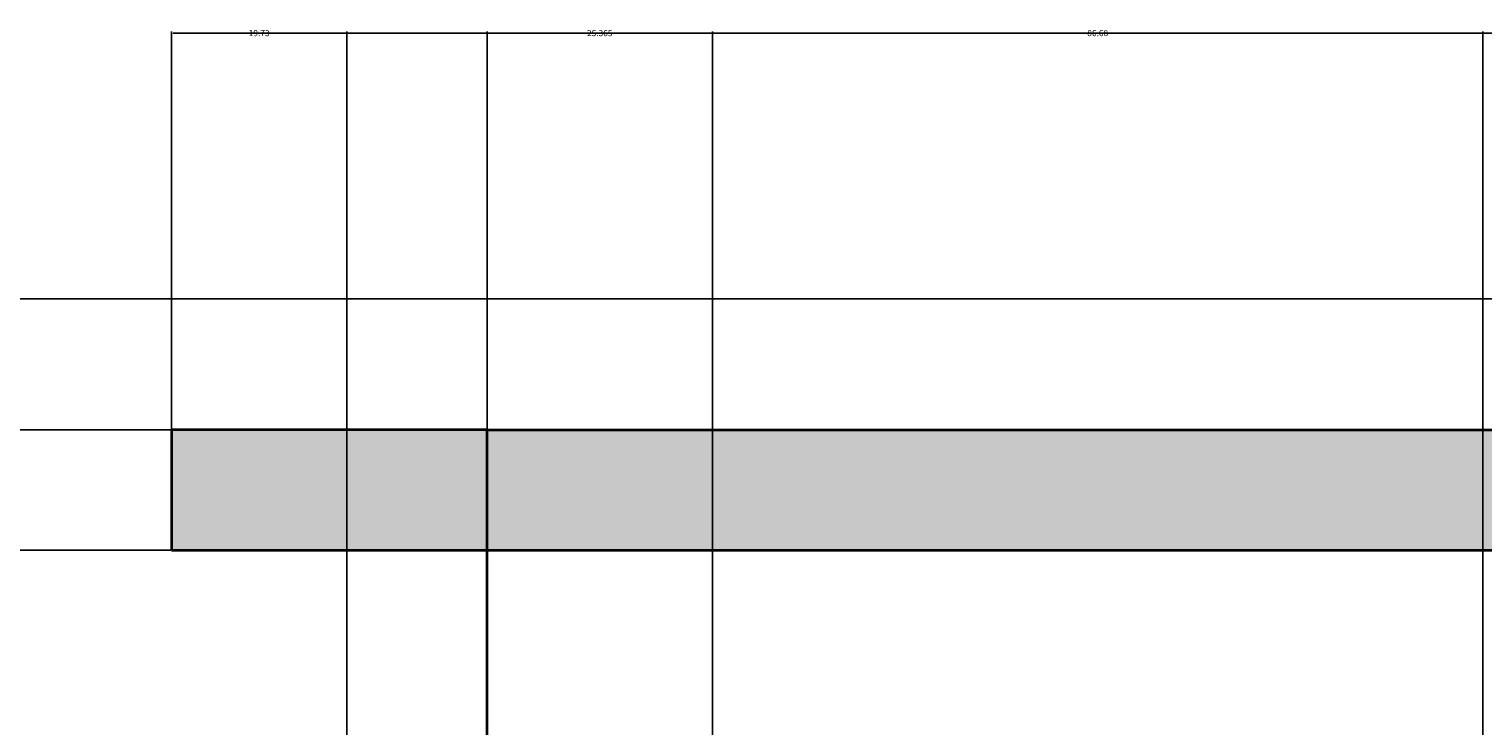
# Model space of a CAD drawing. Units: inches. Extents: x -145 to 510, y 5 to 386.
# Tile 13 of 25: x 18 to 182, y 308 to 386. Entities that reach past the tile are written whole.
import ezdxf

# ---------------------------------------------------------------- set-up
doc = ezdxf.new("R2010")
doc.units = ezdxf.units.IN
doc.header["$MEASUREMENT"] = 0
for name, color, linetype, lineweight in [('A-ANNO-DIMS', 2, 'Continuous', 18), ('A-ELEV', 7, 'Continuous', 35), ('A-ELEV-PATT', 8, 'Continuous', 13)]:
    doc.layers.add(name, color=color, linetype=linetype, lineweight=lineweight)
doc.styles.get("Standard").update_dxf_attribs({"font": 'arial.ttf'})
doc.dimstyles.get("Standard").update_dxf_attribs({"dimtxt": 0.6875, "dimasz": 0.18, "dimexe": 0.18, "dimexo": 0.0625, "dimgap": 0.09, "dimtad": 0, "dimtih": 1, "dimtoh": 1, "dimdec": 4, "dimzin": 0, "dimdsep": 46, "dimlunit": 4, "dimtxsty": 'Standard', "dimcen": 0.09, "dimadec": 0, "dimazin": 0, "dimtfac": 1, "dimtdec": 4, "dimtofl": 0, "dimtmove": 0, "dimatfit": 3, "dimfxl": 1, "dimtolj": 1, "dimtzin": 0, "dimarcsym": 0})

# ---------------------------------------------------------------- blocks, each defined once
blk = doc.blocks.new('*D14')
at = {"layer": 'A-ANNO-DIMS', "color": 0, "lineweight": -2, "transparency": 16777216}
for p, q in [((34.27, 341.23), (34.27, 385.97)), ((34.45, 385.79), (255.28, 385.79)), ((478.65, 385.79), (257.81, 385.79)), ((478.83, 355.95), (478.83, 385.97))]:
    blk.add_line(p, q, dxfattribs=at)
at = {"layer": 'A-ANNO-DIMS', "color": 0, "transparency": 16777216}
for points in [[(34.45, 385.82), (34.45, 385.76), (34.27, 385.79)], [(478.65, 385.82), (478.65, 385.76), (478.83, 385.79)]]:
    blk.add_solid(points, dxfattribs=at)
at = {"layer": 'Defpoints', "color": 0, "transparency": 16777216}
for p in [(478.83, 385.79), (478.83, 355.89), (34.27, 341.17)]:
    blk.add_point(p, dxfattribs=at)
at = {"layer": 'A-ANNO-DIMS', "color": 0, "transparency": 16777216, "insert": (256.55, 385.79), "char_height": 0.688, "attachment_point": 5}
blk.add_mtext('\\A1;444.6', dxfattribs=at)
blk = doc.blocks.new('*D15')
at = {"layer": 'A-ANNO-DIMS', "color": 0, "lineweight": -2, "transparency": 16777216}
for p, q in [((69.78, 199.95), (69.78, 385.97)), ((69.96, 385.79), (80.93, 385.79)), ((94.96, 385.79), (83.98, 385.79)), ((95.14, 305.8), (95.14, 385.97))]:
    blk.add_line(p, q, dxfattribs=at)
at = {"layer": 'A-ANNO-DIMS', "color": 0, "transparency": 16777216}
for points in [[(69.96, 385.82), (69.96, 385.76), (69.78, 385.79)], [(94.96, 385.82), (94.96, 385.76), (95.14, 385.79)]]:
    blk.add_solid(points, dxfattribs=at)
at = {"layer": 'Defpoints', "color": 0, "transparency": 16777216}
for p in [(95.14, 385.79), (95.14, 305.74), (69.78, 199.89)]:
    blk.add_point(p, dxfattribs=at)
at = {"layer": 'A-ANNO-DIMS', "color": 0, "transparency": 16777216, "insert": (82.46, 385.79), "char_height": 0.688, "attachment_point": 5}
blk.add_mtext('\\A1;25.365', dxfattribs=at)
blk = doc.blocks.new('*D16')
at = {"layer": 'A-ANNO-DIMS', "color": 0, "lineweight": -2, "transparency": 16777216}
for p, q in [((95.14, 305.8), (95.14, 385.97)), ((95.32, 385.79), (137.23, 385.79)), ((181.64, 385.79), (139.73, 385.79)), ((181.82, 305.8), (181.82, 385.97))]:
    blk.add_line(p, q, dxfattribs=at)
at = {"layer": 'A-ANNO-DIMS', "color": 0, "transparency": 16777216}
for points in [[(95.32, 385.82), (95.32, 385.76), (95.14, 385.79)], [(181.64, 385.82), (181.64, 385.76), (181.82, 385.79)]]:
    blk.add_solid(points, dxfattribs=at)
at = {"layer": 'Defpoints', "color": 0, "transparency": 16777216}
for p in [(181.82, 385.79), (95.14, 305.74), (181.82, 305.74)]:
    blk.add_point(p, dxfattribs=at)
at = {"layer": 'A-ANNO-DIMS', "color": 0, "transparency": 16777216, "insert": (138.48, 385.79), "char_height": 0.688, "attachment_point": 5}
blk.add_mtext('\\A1;86.68', dxfattribs=at)
blk = doc.blocks.new('*D19')
at = {"layer": 'A-ANNO-DIMS', "color": 0, "lineweight": -2, "transparency": 16777216}
for p, q in [((478.76, 355.89), (-144.05, 355.89)), ((-143.87, 355.71), (-143.87, 218.33)), ((-143.87, 80.07), (-143.87, 217.45)), ((-114.04, 79.89), (-144.05, 79.89))]:
    blk.add_line(p, q, dxfattribs=at)
at = {"layer": 'A-ANNO-DIMS', "color": 0, "transparency": 16777216}
for points in [[(-143.9, 355.71), (-143.84, 355.71), (-143.87, 355.89)], [(-143.9, 80.07), (-143.84, 80.07), (-143.87, 79.89)]]:
    blk.add_solid(points, dxfattribs=at)
at = {"layer": 'Defpoints', "color": 0, "transparency": 16777216}
for p in [(-143.87, 355.89), (478.83, 355.89), (-113.97, 79.89)]:
    blk.add_point(p, dxfattribs=at)
at = {"layer": 'A-ANNO-DIMS', "color": 0, "transparency": 16777216, "insert": (-143.87, 217.89), "char_height": 0.688, "attachment_point": 5}
blk.add_mtext('\\A1;276', dxfattribs=at)
blk = doc.blocks.new('*D21')
at = {"layer": 'A-ANNO-DIMS', "color": 0, "lineweight": -2, "transparency": 16777216}
for p, q in [((34.21, 327.61), (-144.05, 327.61)), ((-143.87, 327.43), (-143.87, 264.19)), ((-143.87, 200.07), (-143.87, 263.31)), ((69.71, 199.89), (-144.05, 199.89))]:
    blk.add_line(p, q, dxfattribs=at)
at = {"layer": 'A-ANNO-DIMS', "color": 0, "transparency": 16777216}
for points in [[(-143.9, 327.43), (-143.84, 327.43), (-143.87, 327.61)], [(-143.9, 200.07), (-143.84, 200.07), (-143.87, 199.89)]]:
    blk.add_solid(points, dxfattribs=at)
at = {"layer": 'Defpoints', "color": 0, "transparency": 16777216}
for p in [(-143.87, 327.61), (34.27, 327.61), (69.78, 199.89)]:
    blk.add_point(p, dxfattribs=at)
at = {"layer": 'A-ANNO-DIMS', "color": 0, "transparency": 16777216, "insert": (-143.87, 263.75), "char_height": 0.688, "attachment_point": 5}
blk.add_mtext('\\A1;127.72', dxfattribs=at)
blk = doc.blocks.new('*D22')
at = {"layer": 'A-ANNO-DIMS', "color": 0, "lineweight": -2, "transparency": 16777216}
for p, q in [((34.21, 341.17), (-144.05, 341.17)), ((-143.87, 340.99), (-143.87, 334.83)), ((-143.87, 327.79), (-143.87, 333.95)), ((34.21, 327.61), (-144.05, 327.61))]:
    blk.add_line(p, q, dxfattribs=at)
at = {"layer": 'A-ANNO-DIMS', "color": 0, "transparency": 16777216}
for points in [[(-143.9, 340.99), (-143.84, 340.99), (-143.87, 341.17)], [(-143.9, 327.79), (-143.84, 327.79), (-143.87, 327.61)]]:
    blk.add_solid(points, dxfattribs=at)
at = {"layer": 'Defpoints', "color": 0, "transparency": 16777216}
for p in [(-143.87, 341.17), (34.27, 341.17), (34.27, 327.61)]:
    blk.add_point(p, dxfattribs=at)
at = {"layer": 'A-ANNO-DIMS', "color": 0, "transparency": 16777216, "insert": (-143.87, 334.39), "char_height": 0.688, "attachment_point": 5}
blk.add_mtext('\\A1;13.559', dxfattribs=at)
blk = doc.blocks.new('*D43')
at = {"layer": 'A-ANNO-DIMS', "color": 0, "lineweight": -2, "transparency": 16777216}
for p, q in [((34.27, 341.23), (34.27, 385.97)), ((34.45, 385.79), (182.84, 385.79)), ((334.26, 385.79), (185.87, 385.79)), ((334.44, 327.67), (334.44, 385.97))]:
    blk.add_line(p, q, dxfattribs=at)
at = {"layer": 'A-ANNO-DIMS', "color": 0, "transparency": 16777216}
for points in [[(34.45, 385.82), (34.45, 385.76), (34.27, 385.79)], [(334.26, 385.82), (334.26, 385.76), (334.44, 385.79)]]:
    blk.add_solid(points, dxfattribs=at)
at = {"layer": 'Defpoints', "color": 0, "transparency": 16777216}
for p in [(334.44, 385.79), (34.27, 341.17), (334.44, 327.61)]:
    blk.add_point(p, dxfattribs=at)
at = {"layer": 'A-ANNO-DIMS', "color": 0, "transparency": 16777216, "insert": (184.36, 385.79), "char_height": 0.688, "attachment_point": 5}
blk.add_mtext('\\A1;300.17', dxfattribs=at)
blk = doc.blocks.new('*D44')
at = {"layer": 'A-ANNO-DIMS', "color": 0, "lineweight": -2, "transparency": 16777216}
for p, q in [((34.27, 327.67), (34.27, 385.97)), ((34.45, 385.79), (42.92, 385.79)), ((53.82, 385.79), (45.35, 385.79)), ((54, 199.95), (54, 385.97))]:
    blk.add_line(p, q, dxfattribs=at)
at = {"layer": 'A-ANNO-DIMS', "color": 0, "transparency": 16777216}
for points in [[(34.45, 385.82), (34.45, 385.76), (34.27, 385.79)], [(53.82, 385.82), (53.82, 385.76), (54, 385.79)]]:
    blk.add_solid(points, dxfattribs=at)
at = {"layer": 'Defpoints', "color": 0, "transparency": 16777216}
for p in [(54, 385.79), (34.27, 327.61), (54, 199.89)]:
    blk.add_point(p, dxfattribs=at)
at = {"layer": 'A-ANNO-DIMS', "color": 0, "transparency": 16777216, "insert": (44.14, 385.79), "char_height": 0.688, "attachment_point": 5}
blk.add_mtext('\\A1;19.73', dxfattribs=at)

msp = doc.modelspace()

# ---------------------------------------------------------------- hatches: boundary and pattern name
at = {"layer": 'A-ELEV-PATT'}
h = msp.add_hatch(color=256, dxfattribs=at)
h.dxf.hatch_style = 1
h.paths.add_polyline_path([(334.4402, 341.168), (69.7763, 341.168), (69.7763, 327.6093), (334.4402, 327.6093)])
h.paths.add_polyline_path([(69.7763, 341.168), (34.2706, 341.168), (34.2706, 327.6093), (69.7763, 327.6093)])
h.paths.add_polyline_path([(317.2273, 188.3087), (210.7973, 188.3087), (210.7973, 178.0195), (317.2273, 178.0195)])
h.paths.add_polyline_path([(474.4893, 235.8905), (317.2273, 235.8905), (317.2273, 223.8905), (474.4893, 223.8905)])
h.paths.add_polyline_path([(317.2273, 235.8905), (309.4739, 235.8905), (309.4739, 223.8905), (317.2273, 223.8905)])
h.paths.add_polyline_path([(478.8263, 235.8905), (474.4893, 235.8905), (474.4893, 223.8905), (478.8263, 223.8905)])

# ---------------------------------------------------------------- linework, layer by layer
at = {"layer": 'A-ELEV'}
for p, q in [((69.7763, 341.168), (34.2706, 341.168)), ((34.2706, 341.168), (34.2706, 327.6093)), ((69.7763, 199.8905), (69.7763, 341.168)), ((69.7763, 341.168), (334.4402, 341.168)), ((34.2706, 327.6093), (334.4402, 327.6093))]:
    msp.add_line(p, q, dxfattribs=at)

# ---------------------------------------------------------------- dimensions: what is measured, and where the dimension line sits
at = {"layer": 'A-ANNO-DIMS'}
for base, p1, p2, override, picture, middle in [((478.8263, 385.7905), (34.2706, 341.168), (478.8263, 355.8905), {"dimdec": 1, "dimlfac": 1, "dimrnd": 0, "dimzin": 0, "dimdsep": 46, "dimlunit": 2}, '*D14', (256.5484, 385.7905)), ((334.4402, 385.7905), (34.2706, 341.168), (334.4402, 327.6093), {"dimdec": 2, "dimlfac": 1, "dimrnd": 0, "dimzin": 0, "dimdsep": 46, "dimlunit": 2}, '*D43', (184.3554, 385.7905)), ((54.0014, 385.7905), (34.2706, 327.6093), (54.0014, 199.8905), {"dimdec": 2, "dimlfac": 1, "dimrnd": 0, "dimzin": 0, "dimdsep": 46, "dimlunit": 2}, '*D44', (44.136, 385.7905)), ((95.1414, 385.7905), (69.7763, 199.8905), (95.1414, 305.7416), {"dimdec": 3, "dimlfac": 1, "dimrnd": 0, "dimzin": 0, "dimdsep": 46, "dimlunit": 2}, '*D15', (82.4589, 385.7905)), ((181.8195, 385.7905), (95.1414, 305.7416), (181.8195, 305.7416), {"dimdec": 2, "dimlfac": 1, "dimrnd": 0, "dimzin": 0, "dimdsep": 46, "dimlunit": 2}, '*D16', (138.4805, 385.7905))]:
    dim = msp.add_linear_dim(base=base, p1=p1, p2=p2, dimstyle='Standard', override=override, dxfattribs=at)
    dim.commit()
    dim.dimension.update_dxf_attribs({"geometry": picture, "text_midpoint": middle})
for base, p1, p2, override, picture, middle in [((-143.8737, 355.8905), (-113.9737, 79.8905), (478.8263, 355.8905), {"dimdec": 0, "dimlfac": 1, "dimrnd": 0, "dimzin": 0, "dimdsep": 46, "dimlunit": 2}, '*D19', (-143.8737, 217.8905)), ((-143.8737, 341.168), (34.2706, 327.6093), (34.2706, 341.168), {"dimdec": 3, "dimlfac": 1, "dimrnd": 0, "dimzin": 0, "dimdsep": 46, "dimlunit": 2}, '*D22', (-143.8737, 334.3886)), ((-143.8737, 327.6093), (69.7763, 199.8905), (34.2706, 327.6093), {"dimdec": 2, "dimlfac": 1, "dimrnd": 0, "dimzin": 0, "dimdsep": 46, "dimlunit": 2}, '*D21', (-143.8737, 263.7499))]:
    dim = msp.add_linear_dim(base=base, p1=p1, p2=p2, angle=90, dimstyle='Standard', override=override, dxfattribs=at)
    dim.commit()
    dim.dimension.update_dxf_attribs({"geometry": picture, "text_midpoint": middle})

doc.saveas('drawing.dxf')
